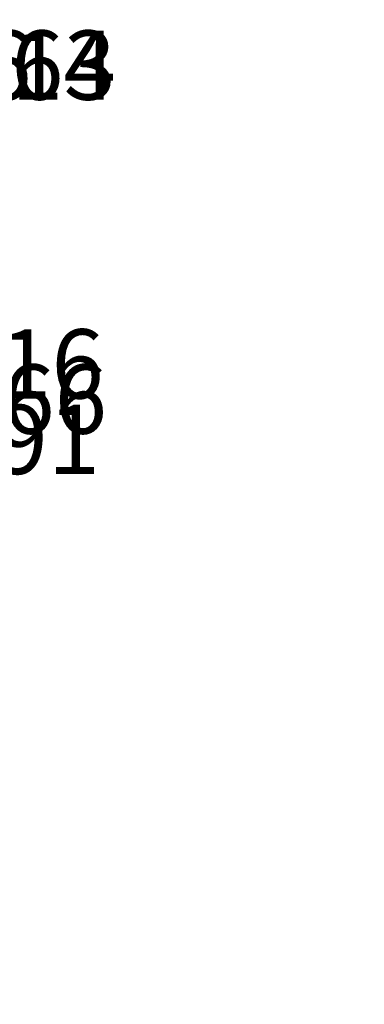
# Model space of a CAD drawing. Units: inches. Extents: x 172 to 828, y 190 to 777.
# Tile 9 of 9: x 708 to 828, y 436 to 777. Entities that reach past the tile are written whole.
import ezdxf

# ---------------------------------------------------------------- set-up
doc = ezdxf.new("R2010")
doc.units = ezdxf.units.IN
doc.header["$MEASUREMENT"] = 0
doc.layers.add('A-ANNO-DIMS', color=2, linetype='Continuous', lineweight=18)
doc.styles.get("Standard").update_dxf_attribs({"font": 'arial.ttf'})
doc.dimstyles.get("Standard").update_dxf_attribs({"dimtxt": 24, "dimasz": 12, "dimexe": 0.18, "dimexo": 0.0625, "dimgap": 0.09, "dimtad": 0, "dimtih": 1, "dimtoh": 1, "dimdec": 0, "dimzin": 0, "dimdsep": 46, "dimlunit": 3, "dimtxsty": 'Standard', "dimcen": 0.09, "dimadec": 0, "dimazin": 0, "dimtfac": 1, "dimtdec": 0, "dimtofl": 0, "dimtmove": 0, "dimatfit": 3, "dimfxl": 1, "dimtolj": 1, "dimtzin": 0, "dimarcsym": 0})

# ---------------------------------------------------------------- blocks, each defined once
blk = doc.blocks.new('*D4')
at = {"layer": 'A-ANNO-DIMS', "color": 0, "lineweight": -2, "transparency": 16777216}
for p, q in [((601.02, 471.8), (617.1, 471.8)), ((616.92, 459.8), (616.92, 431.1)), ((616.92, 377.39), (616.92, 406.09)), ((601.02, 365.39), (617.1, 365.39))]:
    blk.add_line(p, q, dxfattribs=at)
at = {"layer": 'A-ANNO-DIMS', "color": 0, "transparency": 16777216}
for points in [[(614.92, 459.8), (618.92, 459.8), (616.92, 471.8)], [(614.92, 377.39), (618.92, 377.39), (616.92, 365.39)]]:
    blk.add_solid(points, dxfattribs=at)
at = {"layer": 'Defpoints', "color": 0, "transparency": 16777216}
for p in [(600.96, 471.8), (616.92, 471.8), (600.96, 365.39)]:
    blk.add_point(p, dxfattribs=at)
at = {"layer": 'A-ANNO-DIMS', "color": 0, "transparency": 16777216, "insert": (616.92, 418.6), "char_height": 24, "attachment_point": 5}
blk.add_mtext('\\A1;BALCONY WINDOW 106 TYP.', dxfattribs=at)
blk = doc.blocks.new('*D50')
at = {"layer": 'A-ANNO-DIMS', "color": 0, "lineweight": -2, "transparency": 16777216}
for p, q in [((589.47, 761.09), (577.47, 761.09)), ((601.47, 723.23), (601.47, 761.27)), ((618.78, 735.45), (618.78, 761.27)), ((630.78, 761.09), (642.78, 761.09))]:
    blk.add_line(p, q, dxfattribs=at)
at = {"layer": 'A-ANNO-DIMS', "color": 0, "transparency": 16777216}
for points in [[(589.47, 763.09), (589.47, 759.09), (601.47, 761.09)], [(630.78, 763.09), (630.78, 759.09), (618.78, 761.09)]]:
    blk.add_solid(points, dxfattribs=at)
at = {"layer": 'Defpoints', "color": 0, "transparency": 16777216}
for p in [(618.78, 761.09), (618.78, 735.39), (601.47, 723.17)]:
    blk.add_point(p, dxfattribs=at)
at = {"layer": 'A-ANNO-DIMS', "color": 0, "transparency": 16777216, "insert": (691.51, 761.09), "char_height": 24, "attachment_point": 5}
blk.add_mtext('\\A1;17.314', dxfattribs=at)
blk = doc.blocks.new('*D63')
at = {"layer": 'A-ANNO-DIMS', "color": 0, "lineweight": -2, "transparency": 16777216}
for p, q in [((594.82, 761.09), (582.82, 761.09)), ((606.82, 663.45), (606.82, 761.27)), ((618.78, 723.23), (618.78, 761.27)), ((630.78, 761.09), (642.78, 761.09))]:
    blk.add_line(p, q, dxfattribs=at)
at = {"layer": 'A-ANNO-DIMS', "color": 0, "transparency": 16777216}
for points in [[(594.82, 763.09), (594.82, 759.09), (606.82, 761.09)], [(630.78, 763.09), (630.78, 759.09), (618.78, 761.09)]]:
    blk.add_solid(points, dxfattribs=at)
at = {"layer": 'Defpoints', "color": 0, "transparency": 16777216}
for p in [(618.78, 761.09), (618.78, 723.17), (606.82, 663.39)]:
    blk.add_point(p, dxfattribs=at)
at = {"layer": 'A-ANNO-DIMS', "color": 0, "transparency": 16777216, "insert": (691.56, 761.09), "char_height": 24, "attachment_point": 5}
blk.add_mtext('\\A1;11.963', dxfattribs=at)
blk = doc.blocks.new('*D64')
at = {"layer": 'A-ANNO-DIMS', "color": 0, "lineweight": -2, "transparency": 16777216}
for p, q in [((644.98, 645.55), (644.98, 657.55)), ((644.98, 657.55), (656.98, 657.55)), ((518.47, 633.55), (645.16, 633.55)), ((518.47, 615.39), (645.16, 615.39)), ((644.98, 603.39), (644.98, 591.39))]:
    blk.add_line(p, q, dxfattribs=at)
at = {"layer": 'A-ANNO-DIMS', "color": 0, "transparency": 16777216}
for points in [[(642.98, 645.55), (646.98, 645.55), (644.98, 633.55)], [(642.98, 603.39), (646.98, 603.39), (644.98, 615.39)]]:
    blk.add_solid(points, dxfattribs=at)
at = {"layer": 'Defpoints', "color": 0, "transparency": 16777216}
for p in [(518.4, 633.55), (644.98, 633.55), (518.4, 615.39)]:
    blk.add_point(p, dxfattribs=at)
at = {"layer": 'A-ANNO-DIMS', "color": 0, "transparency": 16777216, "insert": (696.43, 657.55), "char_height": 24, "attachment_point": 5}
blk.add_mtext('\\A1;18.16', dxfattribs=at)
blk = doc.blocks.new('*D65')
at = {"layer": 'A-ANNO-DIMS', "color": 0, "lineweight": -2, "transparency": 16777216}
for p, q in [((644.98, 633.36), (644.98, 645.36)), ((644.98, 645.36), (656.98, 645.36)), ((527.16, 621.36), (645.16, 621.36)), ((518.47, 615.39), (645.16, 615.39)), ((644.98, 603.39), (644.98, 591.39))]:
    blk.add_line(p, q, dxfattribs=at)
at = {"layer": 'A-ANNO-DIMS', "color": 0, "transparency": 16777216}
for points in [[(642.98, 633.36), (646.98, 633.36), (644.98, 621.36)], [(642.98, 603.39), (646.98, 603.39), (644.98, 615.39)]]:
    blk.add_solid(points, dxfattribs=at)
at = {"layer": 'Defpoints', "color": 0, "transparency": 16777216}
for p in [(527.09, 621.36), (644.98, 621.36), (518.4, 615.39)]:
    blk.add_point(p, dxfattribs=at)
at = {"layer": 'A-ANNO-DIMS', "color": 0, "transparency": 16777216, "insert": (697.55, 645.36), "char_height": 24, "attachment_point": 5}
blk.add_mtext('\\A1;5.966', dxfattribs=at)
blk = doc.blocks.new('*D82')
at = {"layer": 'A-ANNO-DIMS', "color": 0, "lineweight": -2, "transparency": 16777216}
for p, q in [((588.96, 761.09), (576.96, 761.09)), ((600.96, 493.45), (600.96, 761.27)), ((606.82, 607.45), (606.82, 761.27)), ((618.82, 761.09), (630.82, 761.09))]:
    blk.add_line(p, q, dxfattribs=at)
at = {"layer": 'A-ANNO-DIMS', "color": 0, "transparency": 16777216}
for points in [[(588.96, 763.09), (588.96, 759.09), (600.96, 761.09)], [(618.82, 763.09), (618.82, 759.09), (606.82, 761.09)]]:
    blk.add_solid(points, dxfattribs=at)
at = {"layer": 'Defpoints', "color": 0, "transparency": 16777216}
for p in [(606.82, 761.09), (606.82, 607.39), (600.96, 493.39)]:
    blk.add_point(p, dxfattribs=at)
at = {"layer": 'A-ANNO-DIMS', "color": 0, "transparency": 16777216, "insert": (671.39, 761.09), "char_height": 24, "attachment_point": 5}
blk.add_mtext('\\A1;5.856', dxfattribs=at)
blk = doc.blocks.new('*D91')
at = {"layer": 'A-ANNO-DIMS', "color": 0, "lineweight": -2, "transparency": 16777216}
for p, q in [((644.98, 619.39), (644.98, 631.39)), ((644.98, 631.39), (656.98, 631.39)), ((606.88, 607.39), (645.16, 607.39)), ((591.61, 599.8), (645.16, 599.8)), ((644.98, 587.8), (644.98, 575.8))]:
    blk.add_line(p, q, dxfattribs=at)
at = {"layer": 'A-ANNO-DIMS', "color": 0, "transparency": 16777216}
for points in [[(642.98, 619.39), (646.98, 619.39), (644.98, 607.39)], [(642.98, 587.8), (646.98, 587.8), (644.98, 599.8)]]:
    blk.add_solid(points, dxfattribs=at)
at = {"layer": 'Defpoints', "color": 0, "transparency": 16777216}
for p in [(606.82, 607.39), (644.98, 607.39), (591.54, 599.8)]:
    blk.add_point(p, dxfattribs=at)
at = {"layer": 'A-ANNO-DIMS', "color": 0, "transparency": 16777216, "insert": (695.15, 631.39), "char_height": 24, "attachment_point": 5}
blk.add_mtext('\\A1;7.591', dxfattribs=at)

msp = doc.modelspace()

# ---------------------------------------------------------------- dimensions: what is measured, and where the dimension line sits
at = {"layer": 'A-ANNO-DIMS'}
for base, p1, p2, picture, middle in [((606.8158, 761.0923), (600.9594, 493.3923), (606.8158, 607.3923), '*D82', (671.3915, 761.0923)), ((618.7792, 761.0923), (601.4651, 723.1684), (618.7792, 735.3923), '*D50', (691.5076, 761.0923)), ((618.7792, 761.0923), (606.8158, 663.3923), (618.7792, 723.1684), '*D63', (691.5568, 761.0923))]:
    dim = msp.add_linear_dim(base=base, p1=p1, p2=p2, dimstyle='Standard', override={"dimdec": 3, "dimlfac": 1, "dimrnd": 0, "dimzin": 0, "dimdsep": 46, "dimlunit": 2}, dxfattribs=at)
    dim.commit()
    dim.dimension.update_dxf_attribs({"geometry": picture, "text_midpoint": middle})
for base, p1, p2, override, picture, middle in [((644.9792, 633.5521), (518.4045, 615.3923), (518.4045, 633.5521), {"dimdec": 2, "dimlfac": 1, "dimrnd": 0, "dimzin": 0, "dimdsep": 46, "dimlunit": 2}, '*D64', (696.4252, 657.5521)), ((644.9792, 621.358), (518.4045, 615.3923), (527.0943, 621.358), {"dimdec": 3, "dimlfac": 1, "dimrnd": 0, "dimzin": 0, "dimdsep": 46, "dimlunit": 2}, '*D65', (697.5549, 645.358)), ((644.9792, 607.3923), (591.5446, 599.8013), (606.8158, 607.3923), {"dimdec": 3, "dimlfac": 1, "dimrnd": 0, "dimzin": 0, "dimdsep": 46, "dimlunit": 2}, '*D91', (695.1483, 631.3923))]:
    dim = msp.add_linear_dim(base=base, p1=p1, p2=p2, angle=90, dimstyle='Standard', override=override, dxfattribs=at)
    dim.commit()
    dim.dimension.update_dxf_attribs({"geometry": picture, "text_midpoint": middle})
dim = msp.add_linear_dim(base=(616.9208, 471.8013), p1=(600.9594, 365.3923), p2=(600.9594, 471.8013), angle=90, text='BALCONY WINDOW <> TYP.', dimstyle='Standard', override={"dimdec": 0, "dimlfac": 1, "dimrnd": 0, "dimzin": 0, "dimdsep": 46, "dimlunit": 2}, dxfattribs=at)
dim.commit()
dim.dimension.update_dxf_attribs({"geometry": '*D4', "text_midpoint": (616.9208, 418.5968)})

doc.saveas('drawing.dxf')
